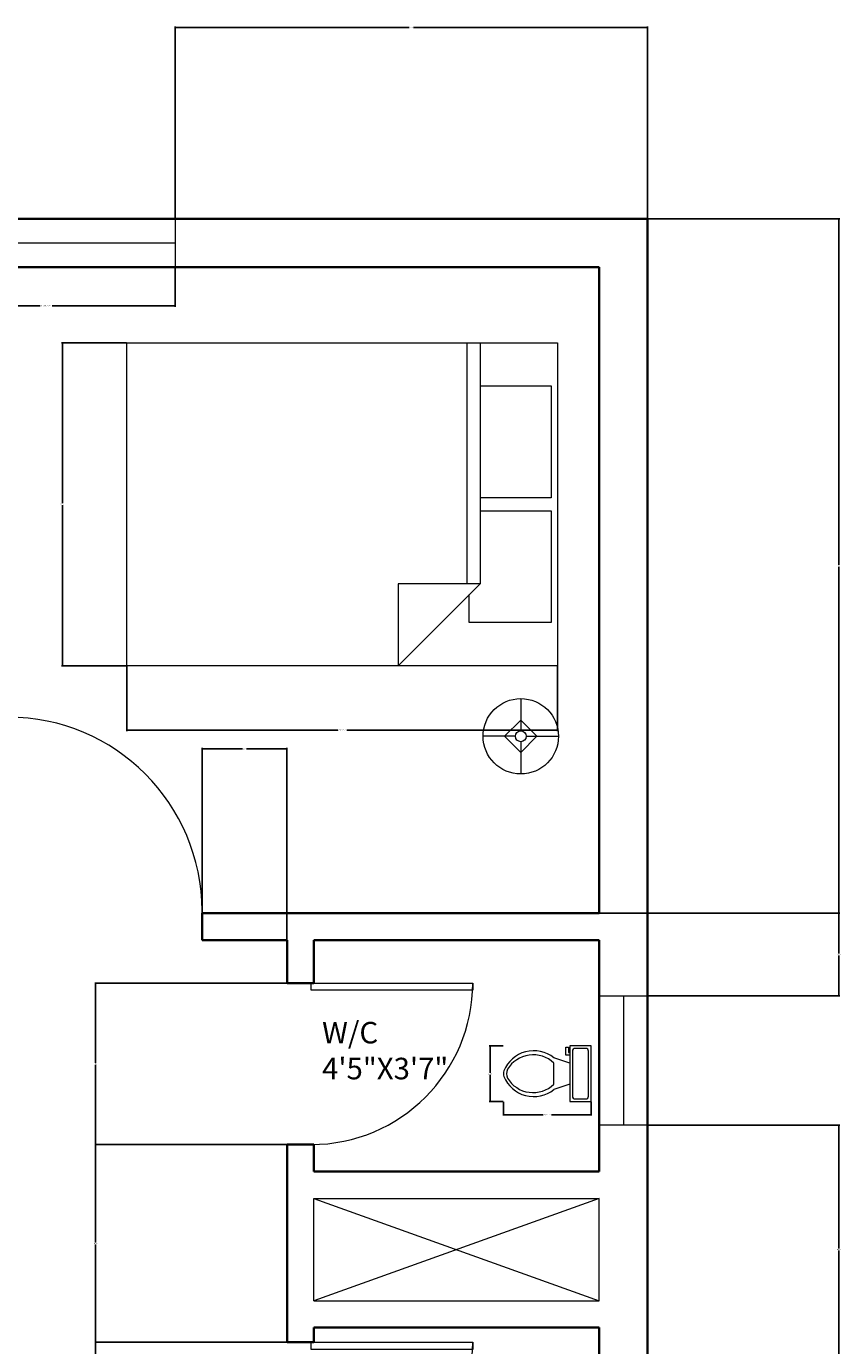
# Model space of a CAD drawing. Units: inches. Extents: x 7766 to 8631, y 9203 to 9940.
# Tile 4 of 6: x 7952 to 8103, y 9695 to 9940. Entities that reach past the tile are written whole.
import ezdxf

# ---------------------------------------------------------------- set-up
doc = ezdxf.new("R2010")
doc.units = ezdxf.units.IN
for name, color, linetype, lineweight in [('A-ANNO-DIMS', 2, 'Continuous', 18), ('A-AREA-IDEN', 11, 'Continuous', 18), ('A-FLOR-FIXT', 9, 'Continuous', 18), ('A-FLOR-OPEN', 7, 'Continuous', 18), ('A-WALL', 7, 'Continuous', 35), ('door', 1, 'Continuous', 18), ('furniture', 6, 'Continuous', 18), ('window', 3, 'Continuous', 18)]:
    doc.layers.add(name, color=color, linetype=linetype, lineweight=lineweight)
doc.styles.get("Standard").update_dxf_attribs({"font": 'arial.ttf'})
doc.dimstyles.get("Standard").update_dxf_attribs({"dimtxt": 0.18, "dimasz": 0.18, "dimexe": 0.18, "dimexo": 0.0625, "dimgap": 0.09, "dimtad": 0, "dimtih": 1, "dimtoh": 1, "dimdec": 4, "dimzin": 0, "dimdsep": 46, "dimtxsty": 'Standard', "dimcen": 0.09, "dimadec": 0, "dimazin": 0, "dimtfac": 1, "dimtdec": 4, "dimtofl": 0, "dimtmove": 0, "dimatfit": 3, "dimfxl": 1, "dimtolj": 1, "dimtzin": 0, "dimarcsym": 0})

# ---------------------------------------------------------------- blocks, each defined once
blk = doc.blocks.new('*U2')
for p, q in [((0, 0), (0, -6)), ((40, 0), (40, -6))]:
    blk.add_line(p, q)
blk.add_lwpolyline([(0, 0), (0, 40), (1.75, 40), (1.75, 0)], close=True)
blk.add_arc((0, 0), 40, 0, 90)
blk = doc.blocks.new('Bed - Queen')
for p, q in [((0, -80.00003), (0, 0)), ((0, 0), (59.99999, 0)), ((59.99999, 0), (59.99999, -80.00003)), ((7.99999, -1.2), (28.79998, -1.2)), ((7.99999, -14.4), (7.99999, -1.2)), ((28.79998, -1.2), (28.79998, -14.4)), ((31.19999, -1.2), (51.99999, -1.2)), ((31.19999, -14.4), (31.19999, -1.2)), ((51.99999, -1.2), (51.99999, -16.4)), ((0, -14.4), (44.8, -14.4)), ((59.99999, -29.6), (44.8, -14.4)), ((44.8, -14.4), (44.8, -29.6)), ((44.8, -16.8), (0, -16.8)), ((51.99999, -16.4), (46.79936, -16.4)), ((44.8, -29.6), (59.99999, -29.6)), ((59.99999, -80.00003), (0, -80.00003))]:
    blk.add_line(p, q)
blk = doc.blocks.new('Lamp - Table')
for p, q in [((0, 7), (0, 1)), ((0, 3), (-3, 0)), ((3, 0), (0, 3)), ((-1, 0), (-7, 0)), ((-3, 0), (0, -3)), ((0, -3), (3, 0)), ((1, 0), (7, 0)), ((0, -1), (0, -7))]:
    blk.add_line(p, q)
for radius in [7, 1]:
    blk.add_circle((0, 0), radius)
blk = doc.blocks.new('Toilet - top')
for p, q in [((9.5, -6), (9.5, -2)), ((-10, -8.5), (-8, -8.5)), ((-10, -9.5), (-10, -8.5)), ((-7, -9.5), (-10, -9.5)), ((-8, -8.5), (-8, -8)), ((-7, -8), (-7, -9.5)), ((-4, -8), (-6, -14)), ((4, -8), (6, -14)), ((4, -14), (-4, -14))]:
    blk.add_line(p, q)
blk.add_lwpolyline([(10.5, -8), (10.5, 0), (-10.5, 0), (-10.5, -8)], close=True)
for points in [[(-9.5, -2), (-9.5, -6)], [(8.5, -1), (-8.5, -1)], [(-8.5, -7), (8.5, -7)]]:
    blk.add_lwpolyline(points)
for centre, radius, start, end in [((-8.62, -1.88), 0.884, 81.8699, 188.1301), ((8.62, -1.88), 0.884, 351.8699, 98.1301), ((-8.62, -6.12), 0.884, 171.8699, 278.1301), ((8.62, -6.12), 0.884, 261.8699, 8.1301), ((3.52, -21.58), 12.17, 141.4691, 247.9714), ((4.2, -21.82), 11.33, 136.3677, 238.9468), ((-3.52, -21.58), 12.17, 292.0284, 38.5307), ((-4.2, -21.82), 11.33, 301.053, 43.6321), ((0, -27.88), 4, 245.7318, 294.2682), ((0, -29), 4, 254.8605, 285.1395)]:
    blk.add_arc(centre, radius, start, end)
blk = doc.blocks.new('WIN-48IN')
blk.add_line((4.5, 48), (4.5, 0))
blk.add_lwpolyline([(0, 48), (9, 48), (9, 0), (0, 0)], close=True)
blk = doc.blocks.new('WIN-24IN')
blk.add_line((4.5, 24), (4.5, 0))
blk.add_lwpolyline([(0, 24), (9, 24), (9, 0), (0, 0)], close=True)
blk = doc.blocks.new('SHAFT-53X19')
for p, q in [((0, 19), (53, 19)), ((0, 0), (0, 19)), ((0, 19), (53, 0)), ((53, 19), (0, 0)), ((53, 0), (53, 19)), ((0, 0), (53, 0))]:
    blk.add_line(p, q)
blk = doc.blocks.new('*D28')
at = {"layer": 'A-ANNO-DIMS', "color": 0, "lineweight": -2, "transparency": 16777216}
for p, q in [((7931.49, 9895.5), (7931.49, 9888.18)), ((7979.49, 9895.5), (7979.49, 9888.18)), ((7931.67, 9888.36), (7954.37, 9888.36)), ((7979.31, 9888.36), (7956.61, 9888.36))]:
    blk.add_line(p, q, dxfattribs=at)
at = {"layer": 'A-ANNO-DIMS', "color": 0, "transparency": 16777216}
for points in [[(7931.67, 9888.39), (7931.67, 9888.33), (7931.49, 9888.36)], [(7979.31, 9888.39), (7979.31, 9888.33), (7979.49, 9888.36)]]:
    blk.add_solid(points, dxfattribs=at)
at = {"layer": 'Defpoints', "color": 0, "transparency": 16777216}
for p in [(7931.49, 9895.56), (7979.49, 9895.56), (7931.49, 9888.36)]:
    blk.add_point(p, dxfattribs=at)
at = {"layer": 'A-ANNO-DIMS', "color": 0, "transparency": 16777216, "insert": (7955.49, 9888.36), "char_height": 0.18, "attachment_point": 5}
blk.add_mtext('\\A1;WINDOW 48 TYP.', dxfattribs=at)
blk = doc.blocks.new('*D32')
at = {"layer": 'A-ANNO-DIMS', "color": 0, "lineweight": -2, "transparency": 16777216}
for p, q in [((8040.45, 9740.5), (8040.45, 9737.94)), ((8056.73, 9740.5), (8056.73, 9737.94)), ((8040.63, 9738.12), (8047.81, 9738.12)), ((8056.55, 9738.12), (8049.36, 9738.12))]:
    blk.add_line(p, q, dxfattribs=at)
at = {"layer": 'A-ANNO-DIMS', "color": 0, "transparency": 16777216}
for points in [[(8040.63, 9738.15), (8040.63, 9738.09), (8040.45, 9738.12)], [(8056.55, 9738.15), (8056.55, 9738.09), (8056.73, 9738.12)]]:
    blk.add_solid(points, dxfattribs=at)
at = {"layer": 'Defpoints', "color": 0, "transparency": 16777216}
for p in [(8040.45, 9740.56), (8056.73, 9740.56), (8056.73, 9738.12)]:
    blk.add_point(p, dxfattribs=at)
at = {"layer": 'A-ANNO-DIMS', "color": 0, "transparency": 16777216, "insert": (8048.59, 9738.12), "char_height": 0.18, "attachment_point": 5}
blk.add_mtext('\\A1;WC 16 TYP.', dxfattribs=at)
blk = doc.blocks.new('*D33')
at = {"layer": 'A-ANNO-DIMS', "color": 0, "lineweight": -2, "transparency": 16777216}
for p, q in [((8040.38, 9750.91), (8037.82, 9750.91)), ((8038, 9750.73), (8038, 9745.92)), ((8038, 9740.74), (8038, 9745.55)), ((8040.38, 9740.56), (8037.82, 9740.56))]:
    blk.add_line(p, q, dxfattribs=at)
at = {"layer": 'A-ANNO-DIMS', "color": 0, "transparency": 16777216}
for points in [[(8037.97, 9750.73), (8038.03, 9750.73), (8038, 9750.91)], [(8037.97, 9740.74), (8038.03, 9740.74), (8038, 9740.56)]]:
    blk.add_solid(points, dxfattribs=at)
at = {"layer": 'Defpoints', "color": 0, "transparency": 16777216}
for p in [(8040.45, 9750.91), (8038, 9740.56), (8040.45, 9740.56)]:
    blk.add_point(p, dxfattribs=at)
at = {"layer": 'A-ANNO-DIMS', "color": 0, "transparency": 16777216, "insert": (8038, 9745.73), "char_height": 0.18, "attachment_point": 5}
blk.add_mtext('\\A1;10 TYP.', dxfattribs=at)
blk = doc.blocks.new('*D36')
at = {"layer": 'A-ANNO-DIMS', "color": 0, "lineweight": -2, "transparency": 16777216}
for p, q in [((7970.51, 9821.46), (7970.51, 9809.35)), ((8050.51, 9821.46), (8050.51, 9809.35)), ((7970.69, 9809.53), (8009.7, 9809.53)), ((8050.33, 9809.53), (8011.33, 9809.53))]:
    blk.add_line(p, q, dxfattribs=at)
at = {"layer": 'A-ANNO-DIMS', "color": 0, "transparency": 16777216}
for points in [[(7970.69, 9809.56), (7970.69, 9809.5), (7970.51, 9809.53)], [(8050.33, 9809.56), (8050.33, 9809.5), (8050.51, 9809.53)]]:
    blk.add_solid(points, dxfattribs=at)
at = {"layer": 'Defpoints', "color": 0, "transparency": 16777216}
for p in [(7970.51, 9821.53), (8050.51, 9821.53), (8050.51, 9809.53)]:
    blk.add_point(p, dxfattribs=at)
at = {"layer": 'A-ANNO-DIMS', "color": 0, "transparency": 16777216, "insert": (8010.51, 9809.53), "char_height": 0.18, "attachment_point": 5}
blk.add_mtext('\\A1;BED 80 TYP.', dxfattribs=at)
blk = doc.blocks.new('*D37')
at = {"layer": 'A-ANNO-DIMS', "color": 0, "lineweight": -2, "transparency": 16777216}
for p, q in [((7970.45, 9881.53), (7958.33, 9881.53)), ((7958.51, 9881.35), (7958.51, 9851.71)), ((7958.51, 9821.71), (7958.51, 9851.34)), ((7970.45, 9821.53), (7958.33, 9821.53))]:
    blk.add_line(p, q, dxfattribs=at)
at = {"layer": 'A-ANNO-DIMS', "color": 0, "transparency": 16777216}
for points in [[(7958.48, 9881.35), (7958.54, 9881.35), (7958.51, 9881.53)], [(7958.48, 9821.71), (7958.54, 9821.71), (7958.51, 9821.53)]]:
    blk.add_solid(points, dxfattribs=at)
at = {"layer": 'Defpoints', "color": 0, "transparency": 16777216}
for p in [(7970.51, 9881.53), (7958.51, 9821.53), (7970.51, 9821.53)]:
    blk.add_point(p, dxfattribs=at)
at = {"layer": 'A-ANNO-DIMS', "color": 0, "transparency": 16777216, "insert": (7958.51, 9851.53), "char_height": 0.18, "attachment_point": 5}
blk.add_mtext('\\A1;60 TYP.', dxfattribs=at)
blk = doc.blocks.new('*D76')
at = {"layer": 'A-ANNO-DIMS', "color": 0, "lineweight": -2, "transparency": 16777216}
for p, q in [((7979.49, 9904.63), (7979.49, 9940.29)), ((8067.24, 9904.63), (8067.24, 9940.29)), ((7979.67, 9940.11), (8022.97, 9940.11)), ((8067.06, 9940.11), (8023.76, 9940.11))]:
    blk.add_line(p, q, dxfattribs=at)
at = {"layer": 'A-ANNO-DIMS', "color": 0, "transparency": 16777216}
for points in [[(7979.67, 9940.14), (7979.67, 9940.08), (7979.49, 9940.11)], [(8067.06, 9940.14), (8067.06, 9940.08), (8067.24, 9940.11)]]:
    blk.add_solid(points, dxfattribs=at)
at = {"layer": 'Defpoints', "color": 0, "transparency": 16777216}
for p in [(8067.24, 9940.11), (7979.49, 9904.56), (8067.24, 9904.56)]:
    blk.add_point(p, dxfattribs=at)
at = {"layer": 'A-ANNO-DIMS', "color": 0, "transparency": 16777216, "insert": (8023.37, 9940.11), "char_height": 0.18, "attachment_point": 5}
blk.add_mtext('\\A1;87.75', dxfattribs=at)
blk = doc.blocks.new('*D84')
at = {"layer": 'A-ANNO-DIMS', "color": 0, "lineweight": -2, "transparency": 16777216}
for p, q in [((8067.31, 9736.18), (8102.97, 9736.18)), ((8102.79, 9736), (8102.79, 9713.23)), ((8102.79, 9690.09), (8102.79, 9712.86)), ((8067.31, 9689.91), (8102.97, 9689.91))]:
    blk.add_line(p, q, dxfattribs=at)
at = {"layer": 'A-ANNO-DIMS', "color": 0, "transparency": 16777216}
for points in [[(8102.76, 9736), (8102.82, 9736), (8102.79, 9736.18)], [(8102.76, 9690.09), (8102.82, 9690.09), (8102.79, 9689.91)]]:
    blk.add_solid(points, dxfattribs=at)
at = {"layer": 'Defpoints', "color": 0, "transparency": 16777216}
for p in [(8067.24, 9736.18), (8102.79, 9736.18), (8067.24, 9689.91)]:
    blk.add_point(p, dxfattribs=at)
at = {"layer": 'A-ANNO-DIMS', "color": 0, "transparency": 16777216, "insert": (8102.79, 9713.05), "char_height": 0.18, "attachment_point": 5}
blk.add_mtext('\\A1;46.27', dxfattribs=at)
blk = doc.blocks.new('*D85')
at = {"layer": 'A-ANNO-DIMS', "color": 0, "lineweight": -2, "transparency": 16777216}
for p, q in [((8058.31, 9775.56), (8102.97, 9775.56)), ((8102.79, 9775.38), (8102.79, 9768.05)), ((8102.79, 9760.36), (8102.79, 9767.69)), ((8067.31, 9760.18), (8102.97, 9760.18))]:
    blk.add_line(p, q, dxfattribs=at)
at = {"layer": 'A-ANNO-DIMS', "color": 0, "transparency": 16777216}
for points in [[(8102.76, 9775.38), (8102.82, 9775.38), (8102.79, 9775.56)], [(8102.76, 9760.36), (8102.82, 9760.36), (8102.79, 9760.18)]]:
    blk.add_solid(points, dxfattribs=at)
at = {"layer": 'Defpoints', "color": 0, "transparency": 16777216}
for p in [(8058.24, 9775.56), (8102.79, 9775.56), (8067.24, 9760.18)]:
    blk.add_point(p, dxfattribs=at)
at = {"layer": 'A-ANNO-DIMS', "color": 0, "transparency": 16777216, "insert": (8102.79, 9767.87), "char_height": 0.18, "attachment_point": 5}
blk.add_mtext('\\A1;15.38', dxfattribs=at)
blk = doc.blocks.new('*D86')
at = {"layer": 'A-ANNO-DIMS', "color": 0, "lineweight": -2, "transparency": 16777216}
for p, q in [((8067.31, 9904.56), (8102.97, 9904.56)), ((8102.79, 9904.38), (8102.79, 9840.25)), ((8102.79, 9775.74), (8102.79, 9839.88)), ((8058.31, 9775.56), (8102.97, 9775.56))]:
    blk.add_line(p, q, dxfattribs=at)
at = {"layer": 'A-ANNO-DIMS', "color": 0, "transparency": 16777216}
for points in [[(8102.76, 9904.38), (8102.82, 9904.38), (8102.79, 9904.56)], [(8102.76, 9775.74), (8102.82, 9775.74), (8102.79, 9775.56)]]:
    blk.add_solid(points, dxfattribs=at)
at = {"layer": 'Defpoints', "color": 0, "transparency": 16777216}
for p in [(8067.24, 9904.56), (8102.79, 9904.56), (8058.24, 9775.56)]:
    blk.add_point(p, dxfattribs=at)
at = {"layer": 'A-ANNO-DIMS', "color": 0, "transparency": 16777216, "insert": (8102.79, 9840.06), "char_height": 0.18, "attachment_point": 5}
blk.add_mtext('\\A1;129', dxfattribs=at)
blk = doc.blocks.new('*D91')
at = {"layer": 'A-ANNO-DIMS', "color": 0, "lineweight": -2, "transparency": 16777216}
for p, q in [((7984.45, 9770.63), (7984.45, 9806.29)), ((7984.63, 9806.11), (7991.96, 9806.11)), ((8000.06, 9806.11), (7992.73, 9806.11)), ((8000.24, 9770.63), (8000.24, 9806.29))]:
    blk.add_line(p, q, dxfattribs=at)
at = {"layer": 'A-ANNO-DIMS', "color": 0, "transparency": 16777216}
for points in [[(7984.63, 9806.14), (7984.63, 9806.08), (7984.45, 9806.11)], [(8000.06, 9806.14), (8000.06, 9806.08), (8000.24, 9806.11)]]:
    blk.add_solid(points, dxfattribs=at)
at = {"layer": 'Defpoints', "color": 0, "transparency": 16777216}
for p in [(8000.24, 9806.11), (7984.45, 9770.56), (8000.24, 9770.56)]:
    blk.add_point(p, dxfattribs=at)
at = {"layer": 'A-ANNO-DIMS', "color": 0, "transparency": 16777216, "insert": (7992.35, 9806.11), "char_height": 0.18, "attachment_point": 5}
blk.add_mtext('\\A1;15.79', dxfattribs=at)
blk = doc.blocks.new('*D92')
at = {"layer": 'A-ANNO-DIMS', "color": 0, "lineweight": -2, "transparency": 16777216}
for p, q in [((8000.18, 9762.58), (7964.51, 9762.58)), ((7964.69, 9762.4), (7964.69, 9747.76)), ((7964.69, 9732.76), (7964.69, 9747.4)), ((8000.18, 9732.58), (7964.51, 9732.58))]:
    blk.add_line(p, q, dxfattribs=at)
at = {"layer": 'A-ANNO-DIMS', "color": 0, "transparency": 16777216}
for points in [[(7964.66, 9762.4), (7964.72, 9762.4), (7964.69, 9762.58)], [(7964.66, 9732.76), (7964.72, 9732.76), (7964.69, 9732.58)]]:
    blk.add_solid(points, dxfattribs=at)
at = {"layer": 'Defpoints', "color": 0, "transparency": 16777216}
for p in [(7964.69, 9762.58), (8000.24, 9762.58), (8000.24, 9732.58)]:
    blk.add_point(p, dxfattribs=at)
at = {"layer": 'A-ANNO-DIMS', "color": 0, "transparency": 16777216, "insert": (7964.69, 9747.58), "char_height": 0.18, "attachment_point": 5}
blk.add_mtext('\\A1;30', dxfattribs=at)
blk = doc.blocks.new('*D93')
at = {"layer": 'A-ANNO-DIMS', "color": 0, "lineweight": -2, "transparency": 16777216}
for p, q in [((8000.18, 9695.83), (7964.51, 9695.83)), ((7964.69, 9695.65), (7964.69, 9681.01)), ((7964.69, 9666.01), (7964.69, 9680.65)), ((8000.18, 9665.83), (7964.51, 9665.83))]:
    blk.add_line(p, q, dxfattribs=at)
at = {"layer": 'A-ANNO-DIMS', "color": 0, "transparency": 16777216}
for points in [[(7964.66, 9695.65), (7964.72, 9695.65), (7964.69, 9695.83)], [(7964.66, 9666.01), (7964.72, 9666.01), (7964.69, 9665.83)]]:
    blk.add_solid(points, dxfattribs=at)
at = {"layer": 'Defpoints', "color": 0, "transparency": 16777216}
for p in [(7964.69, 9695.83), (8000.24, 9695.83), (8000.24, 9665.83)]:
    blk.add_point(p, dxfattribs=at)
at = {"layer": 'A-ANNO-DIMS', "color": 0, "transparency": 16777216, "insert": (7964.69, 9680.83), "char_height": 0.18, "attachment_point": 5}
blk.add_mtext('\\A1;30', dxfattribs=at)
blk = doc.blocks.new('*D94')
at = {"layer": 'A-ANNO-DIMS', "color": 0, "lineweight": -2, "transparency": 16777216}
for p, q in [((8000.18, 9732.58), (7964.51, 9732.58)), ((7964.69, 9732.4), (7964.69, 9714.39)), ((7964.69, 9696.01), (7964.69, 9714.02)), ((8000.18, 9695.83), (7964.51, 9695.83))]:
    blk.add_line(p, q, dxfattribs=at)
at = {"layer": 'A-ANNO-DIMS', "color": 0, "transparency": 16777216}
for points in [[(7964.66, 9732.4), (7964.72, 9732.4), (7964.69, 9732.58)], [(7964.66, 9696.01), (7964.72, 9696.01), (7964.69, 9695.83)]]:
    blk.add_solid(points, dxfattribs=at)
at = {"layer": 'Defpoints', "color": 0, "transparency": 16777216}
for p in [(7964.69, 9732.58), (8000.24, 9732.58), (8000.24, 9695.83)]:
    blk.add_point(p, dxfattribs=at)
at = {"layer": 'A-ANNO-DIMS', "color": 0, "transparency": 16777216, "insert": (7964.69, 9714.2), "char_height": 0.18, "attachment_point": 5}
blk.add_mtext('\\A1;36.75', dxfattribs=at)

msp = doc.modelspace()

# ---------------------------------------------------------------- linework, layer by layer
at = {"layer": 'A-WALL'}
for p, q in [((7802.243, 9904.5631), (8067.243, 9904.5631)), ((8067.243, 9895.5631), (8067.243, 9904.5631)), ((7811.243, 9895.5631), (8058.243, 9895.5631)), ((8058.243, 9775.5631), (8058.243, 9895.5631)), ((8067.243, 9895.5631), (8067.243, 9295.5631)), ((7984.4542, 9775.5631), (8000.243, 9775.5631)), ((8000.243, 9775.5631), (8058.243, 9775.5631)), ((7984.4542, 9770.5631), (8000.243, 9770.5631)), ((8000.243, 9762.5783), (8000.243, 9770.5631)), ((8005.243, 9770.5631), (8058.243, 9770.5631)), ((8005.243, 9762.5783), (8005.243, 9770.5631)), ((8058.243, 9727.5631), (8058.243, 9770.5631)), ((8000.243, 9695.831), (8000.243, 9732.5783)), ((8005.243, 9727.5631), (8005.243, 9732.5783)), ((8005.243, 9727.5631), (8058.243, 9727.5631)), ((8005.243, 9698.5631), (8058.243, 9698.5631)), ((8005.243, 9695.831), (8005.243, 9698.5631)), ((8058.243, 9655.5631), (8058.243, 9698.5631))]:
    msp.add_line(p, q, dxfattribs=at)
for points in [[(7984.4542, 9775.5631), (7984.4542, 9770.5631)], [(8000.243, 9762.5783), (8005.243, 9762.5783)], [(8005.243, 9732.5783), (8000.243, 9732.5783)], [(8000.243, 9695.831), (8005.243, 9695.831)]]:
    msp.add_lwpolyline(points, dxfattribs=at)

# ---------------------------------------------------------------- block references
at = {"layer": 'A-FLOR-FIXT', "xscale": 0.4927007604311352, "yscale": 0.4927007604311352, "zscale": 0.4927007604311352, "rotation": 270}
msp.add_blockref('Toilet - top', (8056.7276, 9745.735), dxfattribs=at)
at = {"layer": 'A-FLOR-OPEN'}
msp.add_blockref('SHAFT-53X19', (8005.243, 9703.563), dxfattribs=at)
at = {"layer": 'door', "xscale": 0.9, "yscale": 0.9, "zscale": 0.9}
msp.add_blockref('*U2', (7948.4542, 9775.9631), dxfattribs=at)
at = {"layer": 'door', "xscale": 0.75, "yscale": 0.75, "zscale": 0.75, "rotation": 270}
for p in [(8004.743, 9762.5783), (8004.743, 9695.831)]:
    msp.add_blockref('*U2', p, dxfattribs=at)
at = {"layer": 'furniture', "rotation": 270}
msp.add_blockref('Bed - Queen', (8050.5136, 9881.5251), dxfattribs=at)
at = {"layer": 'furniture'}
msp.add_blockref('Lamp - Table', (8043.6754, 9808.4143), dxfattribs=at)
at = {"layer": 'window', "rotation": 89.99999999999748}
msp.add_blockref('WIN-48IN', (7979.4895, 9895.5631), dxfattribs=at)
at = {"layer": 'window'}
msp.add_blockref('WIN-24IN', (8058.243, 9736.182), dxfattribs=at)

# ---------------------------------------------------------------- texts
at = {"layer": 'A-AREA-IDEN', "insert": (8006.7614, 9755.3573), "char_height": 4, "attachment_point": 1}
msp.add_mtext_dynamic_manual_height_columns('W/C\\P4\'5"X3\'7"', width=97.347002, gutter_width=18.8909, heights=[0], dxfattribs=at)

# ---------------------------------------------------------------- dimensions: what is measured, and where the dimension line sits
at = {"layer": 'A-ANNO-DIMS'}
dim = msp.add_linear_dim(base=(8067.243, 9940.1131), p1=(7979.4899, 9904.5631), p2=(8067.243, 9904.5631), dimstyle='Standard', override={"dimdec": 2, "dimlfac": 1, "dimrnd": 0, "dimzin": 0, "dimdsep": 46, "dimlunit": 2}, dxfattribs=at)
dim.commit()
dim.dimension.update_dxf_attribs({"geometry": '*D76', "text_midpoint": (8023.3664, 9940.1131)})
for base, p1, p2, angle, override, picture, middle in [((8102.793, 9904.5631), (8058.243, 9775.5631), (8067.243, 9904.5631), 90, {"dimdec": 0, "dimlfac": 1, "dimrnd": 0, "dimzin": 0, "dimdsep": 46, "dimlunit": 2}, '*D86', (8102.793, 9840.0631)), ((8000.243, 9806.1131), (7984.4542, 9770.5631), (8000.243, 9770.5631), 0, {"dimdec": 2, "dimlfac": 1, "dimrnd": 0, "dimzin": 0, "dimdsep": 46, "dimlunit": 2}, '*D91', (7992.3486, 9806.1131)), ((8102.793, 9775.5631), (8067.243, 9760.1825), (8058.243, 9775.5631), 90, {"dimdec": 2, "dimlfac": 1, "dimrnd": 0, "dimzin": 0, "dimdsep": 46, "dimlunit": 2}, '*D85', (8102.793, 9767.8728)), ((7964.693, 9762.5783), (8000.243, 9732.5783), (8000.243, 9762.5783), 90, {"dimdec": 0, "dimlfac": 1, "dimrnd": 0, "dimzin": 0, "dimdsep": 46, "dimlunit": 2}, '*D92', (7964.693, 9747.5783)), ((8102.793, 9736.1825), (8067.243, 9689.9099), (8067.243, 9736.1825), 90, {"dimdec": 2, "dimlfac": 1, "dimrnd": 0, "dimzin": 0, "dimdsep": 46, "dimlunit": 2}, '*D84', (8102.793, 9713.0462)), ((7964.693, 9732.5783), (8000.243, 9695.831), (8000.243, 9732.5783), 90, {"dimdec": 2, "dimlfac": 1, "dimrnd": 0, "dimzin": 0, "dimdsep": 46, "dimlunit": 2}, '*D94', (7964.693, 9714.2046)), ((7964.693, 9695.831), (8000.243, 9665.831), (8000.243, 9695.831), 90, {"dimdec": 0, "dimlfac": 1, "dimrnd": 0, "dimzin": 0, "dimdsep": 46, "dimlunit": 2}, '*D93', (7964.693, 9680.831))]:
    dim = msp.add_linear_dim(base=base, p1=p1, p2=p2, angle=angle, dimstyle='Standard', override=override, dxfattribs=at)
    dim.commit()
    dim.dimension.update_dxf_attribs({"geometry": picture, "text_midpoint": middle})
for base, p1, p2, angle, text, picture, middle in [((7931.4899, 9888.3631), (7979.4899, 9895.5631), (7931.4899, 9895.5631), 180, 'WINDOW <> TYP.', '*D28', (7955.4899, 9888.3631)), ((7958.5136, 9821.5251), (7970.5136, 9881.5251), (7970.5136, 9821.5251), 270, '<> TYP.', '*D37', (7958.5136, 9851.5251)), ((8038.0034, 9740.5616), (8040.4456, 9750.9083), (8040.4456, 9740.5616), 270, '<> TYP.', '*D33', (8038.0034, 9745.735))]:
    dim = msp.add_linear_dim(base=base, p1=p1, p2=p2, angle=angle, text=text, dimstyle='Standard', override={"dimdec": 0, "dimlfac": 1, "dimrnd": 0, "dimzin": 0, "dimdsep": 46, "dimlunit": 2}, dxfattribs=at)
    dim.commit()
    dim.dimension.update_dxf_attribs({"geometry": picture, "text_midpoint": middle})
for base, p1, p2, text, picture, middle in [((8050.5136, 9809.5251), (7970.5136, 9821.5251), (8050.5136, 9821.5251), 'BED <> TYP.', '*D36', (8010.5136, 9809.5251)), ((8056.7276, 9738.1193), (8040.4456, 9740.5616), (8056.7276, 9740.5616), 'WC <> TYP.', '*D32', (8048.5866, 9738.1193))]:
    dim = msp.add_linear_dim(base=base, p1=p1, p2=p2, text=text, dimstyle='Standard', override={"dimdec": 0, "dimlfac": 1, "dimrnd": 0, "dimzin": 0, "dimdsep": 46, "dimlunit": 2}, dxfattribs=at)
    dim.commit()
    dim.dimension.update_dxf_attribs({"geometry": picture, "text_midpoint": middle})

doc.saveas('drawing.dxf')
